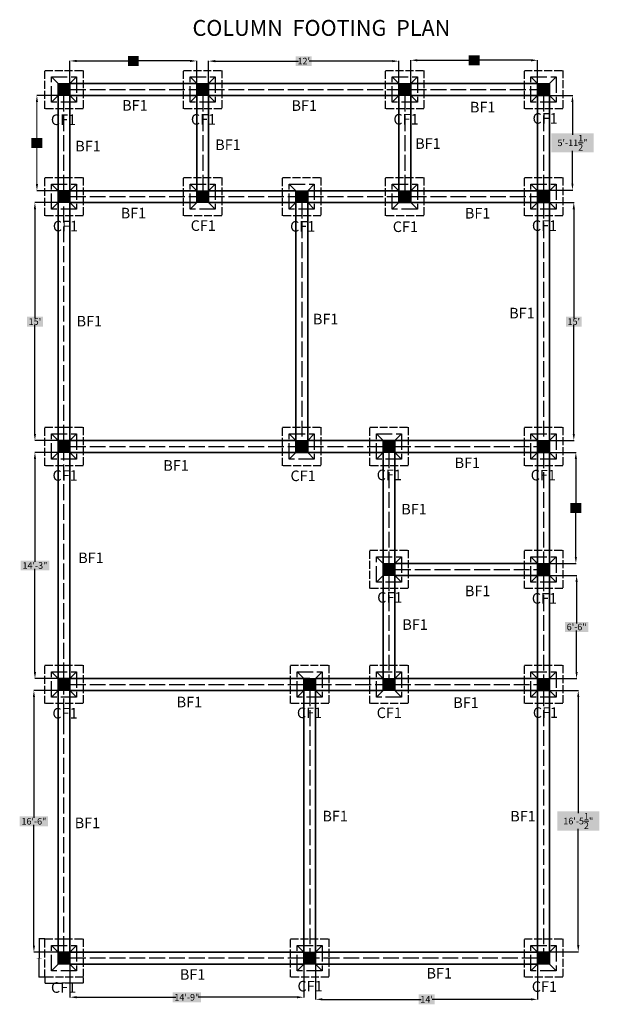
# Model space of a CAD drawing. Units: inches. Extents: x -8 to 1354, y -679 to 94.
# Tile 4 of 6: x 471 to 910, y -666 to 79. Entities that reach past the tile are written whole.
import ezdxf

# ---------------------------------------------------------------- set-up
doc = ezdxf.new("R2010")
doc.units = ezdxf.units.IN
doc.header["$MEASUREMENT"] = 0
doc.linetypes.add('ACAD_ISO02W100', pattern=[15, 12, -3])
for name, color, linetype, lineweight in [('A-ANNO-DIMS', 2, 'Continuous', 18), ('S-ANNO-TEXT', 7, 'Continuous', 25), ('S-BEAM', 152, 'Continuous', 35), ('S-FNDN', 3, 'ACAD_ISO02W100', 25), ('S-FNDN-PATT', 252, 'Continuous', 13)]:
    doc.layers.add(name, color=color, linetype=linetype, lineweight=lineweight)
doc.styles.get("Standard").update_dxf_attribs({"font": 'arial.ttf'})
doc.dimstyles.get("Standard").update_dxf_attribs({"dimtxt": 0.18, "dimasz": 0.18, "dimexe": 0.18, "dimexo": 0.0625, "dimgap": 0.09, "dimtad": 0, "dimtih": 1, "dimtoh": 1, "dimdec": 1, "dimzin": 0, "dimdsep": 46, "dimlunit": 4, "dimtxsty": 'Standard', "dimcen": 0.09, "dimclrd": 2, "dimclre": 3, "dimclrt": 6, "dimadec": 0, "dimazin": 0, "dimtfac": 1, "dimtdec": 1, "dimtofl": 0, "dimtmove": 0, "dimatfit": 3, "dimfxl": 1, "dimtfill": 2, "dimtfillclr": 4, "dimtolj": 1, "dimtzin": 0, "dimarcsym": 0})

# ---------------------------------------------------------------- blocks, each defined once
blk = doc.blocks.new('*D38')
at = {"layer": 'A-ANNO-DIMS', "color": 0, "lineweight": -2, "transparency": 16777216}
for p, q in [((509.02, 21.24), (509.02, 47.49)), ((514.02, 47.31), (554.62, 47.31)), ((600.02, 47.31), (559.41, 47.31)), ((605.02, 21.24), (605.02, 47.49))]:
    blk.add_line(p, q, dxfattribs=at)
at = {"layer": 'A-ANNO-DIMS', "color": 0, "transparency": 16777216}
for points in [[(514.02, 48.15), (514.02, 46.48), (509.02, 47.31)], [(600.02, 48.15), (600.02, 46.48), (605.02, 47.31)]]:
    blk.add_solid(points, dxfattribs=at)
at = {"layer": 'Defpoints', "color": 0, "transparency": 16777216}
for p in [(605.02, 47.31), (509.02, 21.17), (605.02, 21.17)]:
    blk.add_point(p, dxfattribs=at)
at = {"layer": 'A-ANNO-DIMS', "color": 0, "transparency": 16777216, "insert": (557.02, 47.31), "char_height": 5, "attachment_point": 5, "bg_fill": 1, "box_fill_scale": 1.25, "bg_fill_color": 4, "bg_fill_transparency": 0}
blk.add_mtext("\\A1;8'", dxfattribs=at)
blk = doc.blocks.new('*D39')
at = {"layer": 'A-ANNO-DIMS', "color": 0, "lineweight": -2, "transparency": 16777216}
for p, q in [((614.02, 21.24), (614.02, 47.35)), ((619.02, 47.17), (681.92, 47.17)), ((753.02, 47.17), (690.11, 47.17)), ((758.02, 21.24), (758.02, 47.35))]:
    blk.add_line(p, q, dxfattribs=at)
at = {"layer": 'A-ANNO-DIMS', "color": 0, "transparency": 16777216}
for points in [[(619.02, 48), (619.02, 46.33), (614.02, 47.17)], [(753.02, 48), (753.02, 46.33), (758.02, 47.17)]]:
    blk.add_solid(points, dxfattribs=at)
at = {"layer": 'Defpoints', "color": 0, "transparency": 16777216}
for p in [(758.02, 47.17), (614.02, 21.17), (758.02, 21.17)]:
    blk.add_point(p, dxfattribs=at)
at = {"layer": 'A-ANNO-DIMS', "color": 0, "transparency": 16777216, "insert": (686.02, 47.17), "char_height": 5, "attachment_point": 5, "bg_fill": 1, "box_fill_scale": 1.25, "bg_fill_color": 4, "bg_fill_transparency": 0}
blk.add_mtext("\\A1;12'", dxfattribs=at)
blk = doc.blocks.new('*D40')
at = {"layer": 'A-ANNO-DIMS', "color": 0, "lineweight": -2, "transparency": 16777216}
for p, q in [((767.02, 21.24), (767.02, 48.01)), ((772.02, 47.83), (812.62, 47.83)), ((858.02, 47.83), (817.41, 47.83)), ((863.02, 21.24), (863.02, 48.01))]:
    blk.add_line(p, q, dxfattribs=at)
at = {"layer": 'A-ANNO-DIMS', "color": 0, "transparency": 16777216}
for points in [[(772.02, 48.66), (772.02, 46.99), (767.02, 47.83)], [(858.02, 48.66), (858.02, 46.99), (863.02, 47.83)]]:
    blk.add_solid(points, dxfattribs=at)
at = {"layer": 'Defpoints', "color": 0, "transparency": 16777216}
for p in [(863.02, 47.83), (767.02, 21.17), (863.02, 21.17)]:
    blk.add_point(p, dxfattribs=at)
at = {"layer": 'A-ANNO-DIMS', "color": 0, "transparency": 16777216, "insert": (815.02, 47.83), "char_height": 5, "attachment_point": 5, "bg_fill": 1, "box_fill_scale": 1.25, "bg_fill_color": 4, "bg_fill_transparency": 0}
blk.add_mtext("\\A1;8'", dxfattribs=at)
blk = doc.blocks.new('*D41')
at = {"layer": 'A-ANNO-DIMS', "color": 0, "lineweight": -2, "transparency": 16777216}
for p, q in [((508.95, 21.17), (483.84, 21.17)), ((508.95, -50.83), (483.84, -50.83))]:
    blk.add_line(p, q, dxfattribs=at)
at = {"layer": 'A-ANNO-DIMS', "color": 0, "lineweight": 5, "transparency": 16777216}
for p, q in [((484.02, 16.17), (484.02, -12.18)), ((484.02, -45.83), (484.02, -17.47))]:
    blk.add_line(p, q, dxfattribs=at)
at = {"layer": 'A-ANNO-DIMS', "color": 0, "transparency": 16777216}
for points in [[(483.19, 16.17), (484.85, 16.17), (484.02, 21.17)], [(483.19, -45.83), (484.85, -45.83), (484.02, -50.83)]]:
    blk.add_solid(points, dxfattribs=at)
at = {"layer": 'Defpoints', "color": 0, "transparency": 16777216}
for p in [(484.02, 21.17), (509.02, 21.17), (509.02, -50.83)]:
    blk.add_point(p, dxfattribs=at)
at = {"layer": 'A-ANNO-DIMS', "color": 0, "transparency": 16777216, "insert": (484.02, -14.83), "char_height": 5, "attachment_point": 5, "bg_fill": 1, "box_fill_scale": 1.25, "bg_fill_color": 4, "bg_fill_transparency": 0}
blk.add_mtext("\\A1;6'", dxfattribs=at)
blk = doc.blocks.new('*D42')
at = {"layer": 'A-ANNO-DIMS', "color": 0, "lineweight": -2, "transparency": 16777216}
for p, q in [((863.08, 21.17), (889.6, 21.17)), ((889.42, 16.17), (889.42, -8.63)), ((889.42, -45.4), (889.42, -20.6)), ((863.08, -50.4), (889.6, -50.4))]:
    blk.add_line(p, q, dxfattribs=at)
at = {"layer": 'A-ANNO-DIMS', "color": 0, "transparency": 16777216}
for points in [[(888.58, 16.17), (890.25, 16.17), (889.42, 21.17)], [(888.58, -45.4), (890.25, -45.4), (889.42, -50.4)]]:
    blk.add_solid(points, dxfattribs=at)
at = {"layer": 'Defpoints', "color": 0, "transparency": 16777216}
for p in [(863.02, 21.17), (863.02, -50.4), (889.42, -50.4)]:
    blk.add_point(p, dxfattribs=at)
at = {"layer": 'A-ANNO-DIMS', "color": 0, "transparency": 16777216, "insert": (889.42, -14.61), "char_height": 5, "attachment_point": 5, "bg_fill": 1, "box_fill_scale": 1.25, "bg_fill_color": 4, "bg_fill_transparency": 0}
blk.add_mtext('\\A1;5\'-11{\\H1x;\\S1/2;}"', dxfattribs=at)
blk = doc.blocks.new('*D43')
at = {"layer": 'A-ANNO-DIMS', "color": 0, "lineweight": -2, "transparency": 16777216}
for p, q in [((508.95, -59.83), (482.33, -59.83)), ((482.51, -64.83), (482.51, -147.18)), ((482.51, -234.83), (482.51, -152.47)), ((508.95, -239.83), (482.33, -239.83))]:
    blk.add_line(p, q, dxfattribs=at)
at = {"layer": 'A-ANNO-DIMS', "color": 0, "transparency": 16777216}
for points in [[(481.68, -64.83), (483.34, -64.83), (482.51, -59.83)], [(481.68, -234.83), (483.34, -234.83), (482.51, -239.83)]]:
    blk.add_solid(points, dxfattribs=at)
at = {"layer": 'Defpoints', "color": 0, "transparency": 16777216}
for p in [(509.02, -59.83), (482.51, -239.83), (509.02, -239.83)]:
    blk.add_point(p, dxfattribs=at)
at = {"layer": 'A-ANNO-DIMS', "color": 0, "transparency": 16777216, "insert": (482.51, -149.83), "char_height": 5, "attachment_point": 5, "bg_fill": 1, "box_fill_scale": 1.25, "bg_fill_color": 4, "bg_fill_transparency": 0}
blk.add_mtext("\\A1;15'", dxfattribs=at)
blk = doc.blocks.new('*D44')
at = {"layer": 'A-ANNO-DIMS', "color": 0, "lineweight": -2, "transparency": 16777216}
for p, q in [((863.08, -59.83), (890.63, -59.83)), ((890.45, -64.83), (890.45, -147.18)), ((890.45, -234.83), (890.45, -152.47)), ((863.08, -239.83), (890.63, -239.83))]:
    blk.add_line(p, q, dxfattribs=at)
at = {"layer": 'A-ANNO-DIMS', "color": 0, "transparency": 16777216}
for points in [[(889.61, -64.83), (891.28, -64.83), (890.45, -59.83)], [(889.61, -234.83), (891.28, -234.83), (890.45, -239.83)]]:
    blk.add_solid(points, dxfattribs=at)
at = {"layer": 'Defpoints', "color": 0, "transparency": 16777216}
for p in [(863.02, -59.83), (863.02, -239.83), (890.45, -239.83)]:
    blk.add_point(p, dxfattribs=at)
at = {"layer": 'A-ANNO-DIMS', "color": 0, "transparency": 16777216, "insert": (890.45, -149.83), "char_height": 5, "attachment_point": 5, "bg_fill": 1, "box_fill_scale": 1.25, "bg_fill_color": 4, "bg_fill_transparency": 0}
blk.add_mtext("\\A1;15'", dxfattribs=at)
blk = doc.blocks.new('*D45')
at = {"layer": 'A-ANNO-DIMS', "color": 0, "lineweight": -2, "transparency": 16777216}
for p, q in [((863.08, -248.83), (892.19, -248.83)), ((892.01, -253.83), (892.01, -288.24)), ((892.01, -327.83), (892.01, -293.42)), ((863.08, -332.83), (892.19, -332.83))]:
    blk.add_line(p, q, dxfattribs=at)
at = {"layer": 'A-ANNO-DIMS', "color": 0, "transparency": 16777216}
for points in [[(891.18, -253.83), (892.85, -253.83), (892.01, -248.83)], [(891.18, -327.83), (892.85, -327.83), (892.01, -332.83)]]:
    blk.add_solid(points, dxfattribs=at)
at = {"layer": 'Defpoints', "color": 0, "transparency": 16777216}
for p in [(863.02, -248.83), (863.02, -332.83), (892.01, -332.83)]:
    blk.add_point(p, dxfattribs=at)
at = {"layer": 'A-ANNO-DIMS', "color": 0, "transparency": 16777216, "insert": (892.01, -290.83), "char_height": 5, "attachment_point": 5, "bg_fill": 1, "box_fill_scale": 1.25, "bg_fill_color": 4, "bg_fill_transparency": 0}
blk.add_mtext("\\A1;7'", dxfattribs=at)
blk = doc.blocks.new('*D46')
at = {"layer": 'A-ANNO-DIMS', "color": 0, "lineweight": -2, "transparency": 16777216}
for p, q in [((863.08, -341.83), (892.75, -341.83)), ((892.57, -346.83), (892.57, -378.18)), ((892.57, -414.83), (892.57, -383.47)), ((863.08, -419.83), (892.75, -419.83))]:
    blk.add_line(p, q, dxfattribs=at)
at = {"layer": 'A-ANNO-DIMS', "color": 0, "transparency": 16777216}
for points in [[(891.73, -346.83), (893.4, -346.83), (892.57, -341.83)], [(891.73, -414.83), (893.4, -414.83), (892.57, -419.83)]]:
    blk.add_solid(points, dxfattribs=at)
at = {"layer": 'Defpoints', "color": 0, "transparency": 16777216}
for p in [(863.02, -341.83), (892.57, -341.83), (863.02, -419.83)]:
    blk.add_point(p, dxfattribs=at)
at = {"layer": 'A-ANNO-DIMS', "color": 0, "transparency": 16777216, "insert": (892.57, -380.83), "char_height": 5, "attachment_point": 5, "bg_fill": 1, "box_fill_scale": 1.25, "bg_fill_color": 4, "bg_fill_transparency": 0}
blk.add_mtext('\\A1;6\'-6"', dxfattribs=at)
blk = doc.blocks.new('*D47')
at = {"layer": 'A-ANNO-DIMS', "color": 0, "lineweight": -2, "transparency": 16777216}
for p, q in [((863.08, -428.83), (894, -428.83)), ((893.82, -433.83), (893.82, -521.69)), ((893.82, -621.52), (893.82, -533.66)), ((863.08, -626.52), (894, -626.52))]:
    blk.add_line(p, q, dxfattribs=at)
at = {"layer": 'A-ANNO-DIMS', "color": 0, "transparency": 16777216}
for points in [[(892.98, -433.83), (894.65, -433.83), (893.82, -428.83)], [(892.98, -621.52), (894.65, -621.52), (893.82, -626.52)]]:
    blk.add_solid(points, dxfattribs=at)
at = {"layer": 'Defpoints', "color": 0, "transparency": 16777216}
for p in [(863.02, -428.83), (863.02, -626.52), (893.82, -626.52)]:
    blk.add_point(p, dxfattribs=at)
at = {"layer": 'A-ANNO-DIMS', "color": 0, "transparency": 16777216, "insert": (893.82, -527.67), "char_height": 5, "attachment_point": 5, "bg_fill": 1, "box_fill_scale": 1.25, "bg_fill_color": 4, "bg_fill_transparency": 0}
blk.add_mtext('\\A1;16\'-5{\\H1x;\\S1/2;}"', dxfattribs=at)
blk = doc.blocks.new('*D48')
at = {"layer": 'A-ANNO-DIMS', "color": 0, "lineweight": -2, "transparency": 16777216}
for p, q in [((508.95, -248.83), (482.35, -248.83)), ((482.53, -253.83), (482.53, -331.68)), ((482.53, -414.83), (482.53, -336.97)), ((508.95, -419.83), (482.35, -419.83))]:
    blk.add_line(p, q, dxfattribs=at)
at = {"layer": 'A-ANNO-DIMS', "color": 0, "transparency": 16777216}
for points in [[(481.69, -253.83), (483.36, -253.83), (482.53, -248.83)], [(481.69, -414.83), (483.36, -414.83), (482.53, -419.83)]]:
    blk.add_solid(points, dxfattribs=at)
at = {"layer": 'Defpoints', "color": 0, "transparency": 16777216}
for p in [(509.02, -248.83), (482.53, -419.83), (509.02, -419.83)]:
    blk.add_point(p, dxfattribs=at)
at = {"layer": 'A-ANNO-DIMS', "color": 0, "transparency": 16777216, "insert": (482.53, -334.33), "char_height": 5, "attachment_point": 5, "bg_fill": 1, "box_fill_scale": 1.25, "bg_fill_color": 4, "bg_fill_transparency": 0}
blk.add_mtext('\\A1;14\'-3"', dxfattribs=at)
blk = doc.blocks.new('*D49')
at = {"layer": 'A-ANNO-DIMS', "color": 0, "lineweight": -2, "transparency": 16777216}
for p, q in [((508.95, -428.83), (481.56, -428.83)), ((481.74, -433.83), (481.74, -525.18)), ((481.74, -621.83), (481.74, -530.47)), ((508.95, -626.83), (481.56, -626.83))]:
    blk.add_line(p, q, dxfattribs=at)
at = {"layer": 'A-ANNO-DIMS', "color": 0, "transparency": 16777216}
for points in [[(480.91, -433.83), (482.57, -433.83), (481.74, -428.83)], [(480.91, -621.83), (482.57, -621.83), (481.74, -626.83)]]:
    blk.add_solid(points, dxfattribs=at)
at = {"layer": 'Defpoints', "color": 0, "transparency": 16777216}
for p in [(509.02, -428.83), (481.74, -626.83), (509.02, -626.83)]:
    blk.add_point(p, dxfattribs=at)
at = {"layer": 'A-ANNO-DIMS', "color": 0, "transparency": 16777216, "insert": (481.74, -527.83), "char_height": 5, "attachment_point": 5, "bg_fill": 1, "box_fill_scale": 1.25, "bg_fill_color": 4, "bg_fill_transparency": 0}
blk.add_mtext('\\A1;16\'-6"', dxfattribs=at)
blk = doc.blocks.new('*D50')
at = {"layer": 'A-ANNO-DIMS', "color": 0, "lineweight": -2, "transparency": 16777216}
for p, q in [((509.02, -626.89), (509.02, -661.09)), ((686.02, -626.89), (686.02, -661.09)), ((514.02, -660.91), (589.07, -660.91)), ((681.02, -660.91), (605.96, -660.91))]:
    blk.add_line(p, q, dxfattribs=at)
at = {"layer": 'A-ANNO-DIMS', "color": 0, "transparency": 16777216}
for points in [[(514.02, -660.07), (514.02, -661.74), (509.02, -660.91)], [(681.02, -660.07), (681.02, -661.74), (686.02, -660.91)]]:
    blk.add_solid(points, dxfattribs=at)
at = {"layer": 'Defpoints', "color": 0, "transparency": 16777216}
for p in [(509.02, -626.83), (686.02, -626.83), (686.02, -660.91)]:
    blk.add_point(p, dxfattribs=at)
at = {"layer": 'A-ANNO-DIMS', "color": 0, "transparency": 16777216, "insert": (597.52, -660.91), "char_height": 5, "attachment_point": 5, "bg_fill": 1, "box_fill_scale": 1.25, "bg_fill_color": 4, "bg_fill_transparency": 0}
blk.add_mtext('\\A1;14\'-9"', dxfattribs=at)
blk = doc.blocks.new('*D51')
at = {"layer": 'A-ANNO-DIMS', "color": 0, "lineweight": -2, "transparency": 16777216}
for p, q in [((695.02, -626.89), (695.02, -662.7)), ((863.02, -626.89), (863.02, -662.7))]:
    blk.add_line(p, q, dxfattribs=at)
at = {"layer": 'A-ANNO-DIMS', "color": 0, "lineweight": 25, "transparency": 16777216}
for p, q in [((700.02, -662.52), (774.92, -662.52)), ((858.02, -662.52), (783.11, -662.52))]:
    blk.add_line(p, q, dxfattribs=at)
at = {"layer": 'A-ANNO-DIMS', "color": 0, "transparency": 16777216}
for points in [[(700.02, -661.68), (700.02, -663.35), (695.02, -662.52)], [(858.02, -661.68), (858.02, -663.35), (863.02, -662.52)]]:
    blk.add_solid(points, dxfattribs=at)
at = {"layer": 'Defpoints', "color": 0, "transparency": 16777216}
for p in [(695.02, -626.83), (863.02, -626.83), (863.02, -662.52)]:
    blk.add_point(p, dxfattribs=at)
at = {"layer": 'A-ANNO-DIMS', "color": 0, "transparency": 16777216, "insert": (779.02, -662.52), "char_height": 5, "attachment_point": 5, "bg_fill": 1, "box_fill_scale": 1.25, "bg_fill_color": 4, "bg_fill_transparency": 0}
blk.add_mtext("\\A1;14'", dxfattribs=at)
blk = doc.blocks.new('COLUMN-FOOTING-CF1')
at = {"ltscale": 0.5}
for p, q in [((0, 0), (0, 29)), ((0, 29), (29, 29)), ((29, 29), (29, 0)), ((29, 0), (0, 0))]:
    blk.add_line(p, q, dxfattribs=at)
for p, q in [((5, 5), (5, 24)), ((5, 24), (24, 24)), ((10, 19), (5, 24)), ((19, 19), (24, 24)), ((24, 24), (24, 5)), ((10, 10), (10, 19)), ((10, 19), (19, 19)), ((19, 19), (19, 10)), ((5, 5), (10, 10)), ((19, 10), (10, 10)), ((24, 5), (19, 10)), ((24, 5), (5, 5))]:
    blk.add_line(p, q)
blk = doc.blocks.new('*D77')
at = {"layer": 'A-ANNO-DIMS', "color": 3, "lineweight": -2, "transparency": 16777216}
for p, q in [((489.95, -616.83), (485.49, -616.83)), ((489.95, -645.83), (485.49, -645.83))]:
    blk.add_line(p, q, dxfattribs=at)
at = {"layer": 'A-ANNO-DIMS', "color": 2, "lineweight": -2, "transparency": 16777216}
for p, q in [((485.67, -617.01), (485.67, -631.14)), ((485.67, -645.65), (485.67, -631.51))]:
    blk.add_line(p, q, dxfattribs=at)
at = {"layer": 'A-ANNO-DIMS', "color": 2, "transparency": 16777216}
for points in [[(485.64, -617.01), (485.7, -617.01), (485.67, -616.83)], [(485.64, -645.65), (485.7, -645.65), (485.67, -645.83)]]:
    blk.add_solid(points, dxfattribs=at)
at = {"layer": 'Defpoints', "color": 0, "transparency": 16777216}
for p in [(490.02, -616.83), (485.67, -645.83), (490.02, -645.83)]:
    blk.add_point(p, dxfattribs=at)
at = {"layer": 'A-ANNO-DIMS', "color": 6, "transparency": 16777216, "insert": (485.67, -631.33), "char_height": 0.18, "attachment_point": 5, "bg_fill": 1, "box_fill_scale": 1.25, "bg_fill_color": 4, "bg_fill_transparency": 0}
blk.add_mtext('\\A1;COLUMN FOOTING CF1 2\'-5" TYP.', dxfattribs=at)
blk = doc.blocks.new('*D78')
at = {"layer": 'A-ANNO-DIMS', "color": 3, "lineweight": -2, "transparency": 16777216}
for p, q in [((490.02, -645.89), (490.02, -650.36)), ((519.02, -645.89), (519.02, -650.36))]:
    blk.add_line(p, q, dxfattribs=at)
at = {"layer": 'A-ANNO-DIMS', "color": 2, "lineweight": -2, "transparency": 16777216}
for p, q in [((490.2, -650.18), (503.88, -650.18)), ((518.84, -650.18), (505.16, -650.18))]:
    blk.add_line(p, q, dxfattribs=at)
at = {"layer": 'A-ANNO-DIMS', "color": 2, "transparency": 16777216}
for points in [[(490.2, -650.15), (490.2, -650.21), (490.02, -650.18)], [(518.84, -650.15), (518.84, -650.21), (519.02, -650.18)]]:
    blk.add_solid(points, dxfattribs=at)
at = {"layer": 'Defpoints', "color": 0, "transparency": 16777216}
for p in [(490.02, -645.83), (519.02, -645.83), (519.02, -650.18)]:
    blk.add_point(p, dxfattribs=at)
at = {"layer": 'A-ANNO-DIMS', "color": 6, "transparency": 16777216, "insert": (504.52, -650.18), "char_height": 0.18, "attachment_point": 5, "bg_fill": 1, "box_fill_scale": 1.25, "bg_fill_color": 4, "bg_fill_transparency": 0}
blk.add_mtext('\\A1;2\'-5" TYP.', dxfattribs=at)

msp = doc.modelspace()

# ---------------------------------------------------------------- hatches: boundary and pattern name
at = {"layer": 'S-FNDN-PATT'}
h = msp.add_hatch(dxfattribs=at)
h.set_pattern_fill('ANSI31', color=256)
h.set_pattern_definition([(45, (-15.72023, 0), (-0.088388348, 0.088388348), [])])
h.paths.add_polyline_path([(509.02, 30.17), (500.02, 30.17), (500.02, 21.17), (509.02, 21.17)])
h.paths.add_polyline_path([(614.02, 30.17), (605.02, 30.17), (605.02, 21.17), (614.02, 21.17)])
h.paths.add_polyline_path([(767.02, 30.17), (758.02, 30.17), (758.02, 21.17), (767.02, 21.17)])
h.paths.add_polyline_path([(863.02, 30.17), (863.02, 21.17), (872.02, 21.17), (872.02, 30.17)])
h.paths.add_polyline_path([(509.02, -59.83), (509.02, -50.83), (500.02, -50.83), (500.02, -59.83)])
h.paths.add_polyline_path([(605.02, -59.83), (614.02, -59.83), (614.02, -50.83), (605.02, -50.83)])
h.paths.add_polyline_path([(689.02, -50.83), (680.02, -50.83), (680.02, -59.83), (689.02, -59.83)])
h.paths.add_polyline_path([(767.02, -50.83), (758.02, -50.83), (758.02, -59.83), (767.02, -59.83)])
h.paths.add_polyline_path([(863.02, -59.83), (872.02, -59.83), (872.02, -50.83), (863.02, -50.83)])
h.paths.add_polyline_path([(500.02, -248.83), (509.02, -248.83), (509.02, -239.83), (500.02, -239.83)])
h.paths.add_polyline_path([(680.02, -239.83), (680.02, -248.83), (689.02, -248.83), (689.02, -239.83)])
h.paths.add_polyline_path([(746.02, -239.83), (746.02, -248.83), (755.02, -248.83), (755.02, -239.83)])
h.paths.add_polyline_path([(872.02, -248.83), (872.02, -239.83), (863.02, -239.83), (863.02, -248.83)])
h.paths.add_polyline_path([(746.02, -332.83), (746.02, -341.83), (755.02, -341.83), (755.02, -332.83)])
h.paths.add_polyline_path([(863.02, -332.83), (863.02, -341.83), (872.02, -341.83), (872.02, -332.83)])
h.paths.add_polyline_path([(863.02, -428.83), (872.02, -428.83), (872.02, -419.83), (863.02, -419.83)])
h.paths.add_polyline_path([(755.02, -419.83), (746.02, -419.83), (746.02, -428.83), (755.02, -428.83)])
h.paths.add_polyline_path([(695.02, -419.83), (686.02, -419.83), (686.02, -428.83), (695.02, -428.83)])
h.paths.add_polyline_path([(509.02, -419.83), (500.02, -419.83), (500.02, -428.83), (509.02, -428.83)])
h.paths.add_polyline_path([(500.02, -626.83), (500.02, -635.83), (509.02, -635.83), (509.02, -626.83)])
h.paths.add_polyline_path([(695.02, -626.83), (686.02, -626.83), (686.02, -635.83), (695.02, -635.83)])
h.paths.add_polyline_path([(863.02, -626.83), (863.02, -635.83), (872.02, -635.83), (872.02, -626.83)])

# ---------------------------------------------------------------- linework, layer by layer
at = {"layer": 'S-BEAM'}
for p, q in [((509.02, 30.17), (605.02, 30.17)), ((614.02, 30.17), (758.02, 30.17)), ((767.02, 30.17), (863.02, 30.17)), ((500.02, -50.83), (500.02, 21.17)), ((509.02, 21.17), (605.02, 21.17)), ((509.02, -50.83), (509.02, 21.17)), ((605.02, 21.17), (605.02, -50.83)), ((614.02, 21.17), (614.02, -50.83)), ((614.02, 21.17), (758.02, 21.17)), ((758.02, 21.17), (758.02, -50.83)), ((767.02, 21.17), (767.02, -50.83)), ((767.02, 21.17), (863.02, 21.17)), ((863.02, 21.17), (863.02, -50.83)), ((872.02, 21.17), (872.02, -239.83)), ((872.02, 21.17), (872.02, -50.83)), ((605.02, -50.83), (509.02, -50.83)), ((680.02, -50.83), (614.02, -50.83)), ((758.02, -50.83), (689.02, -50.83)), ((863.02, -50.83), (767.02, -50.83)), ((500.02, -59.83), (500.02, -635.83)), ((605.02, -59.83), (509.02, -59.83)), ((509.02, -59.83), (509.02, -239.83)), ((680.02, -59.83), (614.02, -59.83)), ((680.02, -239.83), (680.02, -59.83)), ((767.02, -59.83), (689.02, -59.83)), ((689.02, -239.83), (689.02, -59.83)), ((863.02, -59.83), (767.02, -59.83)), ((863.02, -59.83), (863.02, -239.83)), ((509.02, -239.83), (680.02, -239.83)), ((689.02, -239.83), (863.02, -239.83)), ((509.02, -248.83), (509.02, -419.83)), ((509.02, -248.83), (554.02, -248.83)), ((684.52, -248.83), (509.02, -248.83)), ((554.02, -248.83), (640.47, -248.83)), ((746.02, -248.83), (684.52, -248.83)), ((729.02, -248.83), (746.02, -248.83)), ((746.02, -419.83), (746.02, -248.83)), ((755.02, -248.83), (863.02, -248.83)), ((755.02, -332.83), (755.02, -248.83)), ((863.02, -248.83), (863.02, -332.83)), ((872.02, -248.83), (872.02, -341.83)), ((863.02, -332.83), (755.02, -332.83)), ((755.02, -419.83), (755.02, -341.83)), ((863.02, -341.83), (755.11, -341.83)), ((863.02, -341.83), (863.02, -419.83)), ((872.02, -341.83), (872.02, -428.83)), ((690.52, -419.83), (509.02, -419.83)), ((746.02, -419.83), (695.02, -419.83)), ((863.02, -419.83), (755.11, -419.83)), ((509.02, -428.83), (509.02, -626.83)), ((686.02, -428.83), (509.02, -428.83)), ((686.02, -626.83), (686.02, -428.83)), ((746.02, -428.83), (695.02, -428.83)), ((695.02, -626.83), (695.02, -428.83)), ((863.02, -428.83), (755.02, -428.83)), ((863.02, -428.83), (826.28, -428.83)), ((863.02, -428.83), (863.02, -626.83)), ((872.02, -428.83), (872.02, -626.83)), ((686.02, -626.83), (509.02, -626.83)), ((863.02, -626.83), (695.02, -626.83)), ((686.02, -635.83), (509.02, -635.83)), ((863.02, -635.83), (695.02, -635.83))]:
    msp.add_line(p, q, dxfattribs=at)
at = {"layer": 'S-FNDN'}
for p, q in [((509.02, 25.67), (605.02, 25.67)), ((614.02, 25.67), (758.02, 25.67)), ((767.02, 25.67), (863.02, 25.67)), ((504.52, -50.83), (504.52, 21.17)), ((609.52, 21.17), (609.52, -50.83)), ((762.52, 21.17), (762.52, -50.83)), ((867.52, 21.17), (867.52, -50.83)), ((509.02, -55.33), (605.02, -55.33)), ((614.02, -55.33), (680.02, -55.33)), ((689.02, -55.33), (758.02, -55.33)), ((767.02, -55.33), (863.02, -55.33)), ((504.52, -239.83), (504.52, -59.83)), ((684.52, -59.83), (684.52, -239.83)), ((867.52, -59.83), (867.52, -239.83)), ((509.02, -244.33), (680.02, -244.33)), ((689.02, -244.33), (746.02, -244.33)), ((755.02, -244.33), (863.02, -244.33)), ((504.52, -419.83), (504.52, -248.83)), ((750.52, -248.83), (750.52, -332.83)), ((867.52, -248.83), (867.52, -332.83)), ((750.52, -341.83), (750.52, -419.83)), ((755.02, -337.33), (863.02, -337.33)), ((867.52, -341.83), (867.52, -419.83)), ((509.02, -424.33), (686.02, -424.33)), ((695.02, -424.33), (746.02, -424.33)), ((755.02, -424.33), (863.02, -424.33)), ((504.52, -626.83), (504.52, -428.83)), ((690.52, -428.83), (690.52, -626.83)), ((867.52, -428.83), (867.52, -626.83)), ((686.02, -631.33), (509.02, -631.33)), ((863.02, -631.33), (695.02, -631.33))]:
    msp.add_line(p, q, dxfattribs=at)

# ---------------------------------------------------------------- block references
for p, rotation in [((519.02, 11.17), 89.99999999999935), ((624.02, 11.17), 90), ((777.02, 11.17), 90.00000000000045), ((882.02, 11.17), 90.00000000000067), ((519.02, -40.83), 180), ((595.02, -40.83), 269.9999999999999), ((699.02, -69.83), 90.0000000000003), ((748.02, -40.83), 269.9999999999995), ((519.02, -229.83), 180), ((670.02, -229.83), 269.9999999999996), ((765.02, -258.83), 90.00000000000033), ((882.02, -229.83), 180), ((765.02, -322.83), 179.9941756767035), ((490.02, -409.83), 270.0000000000007), ((705.02, -438.83), 90.00000000000021), ((736.02, -409.82), 269.9941744923129), ((882.02, -409.83), 180), ((490.02, -616.83), 270.0000000000009), ((676.02, -616.83), 269.9999999999993), ((853.02, -616.83), 270)]:
    msp.add_blockref('COLUMN-FOOTING-CF1', p, dxfattribs=dict(at, rotation=rotation))
for p in [(853.02, -69.83), (853.02, -351.83)]:
    msp.add_blockref('COLUMN-FOOTING-CF1', p, dxfattribs=at)

# ---------------------------------------------------------------- texts
at = {"layer": 'S-ANNO-TEXT', "attachment_point": 1}
for s, width, heights, insert, char_height in [('COLUMN  FOOTING  PLAN', 250.6777, [12.42], (601.8, 78.3), 12), ('BF1', 71.0443, [0], (548.56, 17.7), 8), ('BF1', 71.0443, [0], (676.75, 17.55), 8), ('BF1', 71.0443, [0], (811.86, 16.39), 8), ('CF1', 71.0443, [0], (859.22, 7.84), 8), ('CF1', 71.0443, [0], (494.6, 6.85), 8), ('CF1', 71.0443, [0], (600.59, 7.11), 8), ('CF1', 71.0443, [0], (753.9, 7.21), 8), ('BF1', 71.0443, [0], (513.1, -13.09), 8), ('BF1', 71.0443, [0], (619.01, -12.09), 8), ('BF1', 71.0443, [0], (770.4, -11.18), 8), ('BF1', 71.0443, [0], (547.47, -63.77), 8), ('BF1', 71.0443, [0], (808.01, -63.88), 8), ('CF1', 71.0443, [0], (496.08, -73.62), 8), ('CF1', 71.0443, [0], (600.42, -73.25), 8), ('CF1', 71.0443, [0], (675.68, -73.81), 8), ('CF1', 71.0443, [0], (753.42, -74.09), 8), ('CF1', 71.0443, [0], (858.75, -73.27), 8), ('BF1', 71.0443, [0], (841.51, -139.42), 8), ('BF1', 71.0443, [0], (514.06, -145.5), 8), ('BF1', 71.0443, [0], (692.99, -143.92), 8), ('BF1', 71.0443, [0], (800.24, -252.67), 8), ('BF1', 71.0443, [0], (579.73, -254.66), 8), ('CF1', 71.0443, [0], (495.83, -262.26), 8), ('CF1', 71.0443, [0], (675.97, -262.5), 8), ('CF1', 71.0443, [0], (741.25, -261.83), 8), ('CF1', 71.0443, [0], (857.83, -261.99), 8), ('BF1', 71.0443, [0], (759.87, -287.71), 8), ('BF1', 71.0443, [0], (515.26, -324.55), 8), ('BF1', 71.0443, [0], (808.03, -349.58), 8), ('CF1', 71.0443, [0], (741.63, -354.5), 8), ('CF1', 71.0443, [0], (858.66, -355.21), 8), ('BF1', 71.0443, [0], (760.67, -375.02), 8), ('BF1', 71.0443, [0], (589.83, -433.61), 8), ('BF1', 71.0443, [0], (799.23, -434.09), 8), ('CF1', 71.0443, [0], (495.75, -442.1), 8), ('CF1', 71.0443, [0], (680.84, -441.79), 8), ('CF1', 71.0443, [0], (741.25, -441.77), 8), ('CF1', 71.0443, [0], (859.44, -441.63), 8), ('BF1', 71.0443, [0], (700.16, -519.88), 8), ('BF1', 71.0443, [0], (842.38, -519.98), 8), ('BF1', 71.0443, [0], (512.63, -525.05), 8), ('BF1', 71.0443, [0], (592.25, -639.7), 8), ('BF1', 71.0443, [0], (778.94, -638.77), 8), ('CF1', 71.0443, [0], (494.67, -649.56), 8), ('CF1', 71.0443, [0], (681.27, -648.53), 8), ('CF1', 71.0443, [0], (858.65, -648.89), 8)]:
    msp.add_mtext_dynamic_manual_height_columns(s, width=width, gutter_width=1, heights=heights, dxfattribs=dict(at, insert=insert, char_height=char_height))

# ---------------------------------------------------------------- dimensions: what is measured, and where the dimension line sits
at = {"layer": 'A-ANNO-DIMS'}
for base, p1, p2, override, picture, middle in [((605.02, 47.31), (509.02, 21.17), (605.02, 21.17), {"dimtxt": 5, "dimasz": 5, "dimclrd": 0, "dimclre": 0, "dimclrt": 0}, '*D38', (557.02, 47.31)), ((758.02, 47.17), (614.02, 21.17), (758.02, 21.17), {"dimtxt": 5, "dimasz": 5, "dimclrd": 0, "dimclre": 0, "dimclrt": 0}, '*D39', (686.02, 47.17)), ((863.02, 47.83), (767.02, 21.17), (863.02, 21.17), {"dimtxt": 5, "dimasz": 5, "dimclrd": 0, "dimclre": 0, "dimclrt": 0}, '*D40', (815.02, 47.83)), ((686.02, -660.91), (509.02, -626.83), (686.02, -626.83), {"dimtxt": 5, "dimasz": 5, "dimclrd": 0, "dimclre": 0, "dimclrt": 0}, '*D50', (597.52, -660.91)), ((863.02, -662.52), (695.02, -626.83), (863.02, -626.83), {"dimtxt": 5, "dimasz": 5, "dimclrd": 0, "dimclre": 0, "dimclrt": 0, "dimlwd": 25}, '*D51', (779.02, -662.52))]:
    dim = msp.add_linear_dim(base=base, p1=p1, p2=p2, dimstyle='Standard', override=override, dxfattribs=at)
    dim.commit()
    dim.dimension.update_dxf_attribs({"geometry": picture, "text_midpoint": middle})
for base, p1, p2, override, picture, middle in [((484.02, 21.17), (509.02, -50.83), (509.02, 21.17), {"dimtxt": 5, "dimasz": 5, "dimclrd": 0, "dimclre": 0, "dimclrt": 0, "dimlwd": 5}, '*D41', (484.02, -14.83)), ((889.42, -50.4), (863.02, 21.17), (863.02, -50.4), {"dimtxt": 5, "dimasz": 5, "dimclrd": 0, "dimclre": 0, "dimclrt": 0}, '*D42', (889.42, -14.61)), ((482.51, -239.83), (509.02, -59.83), (509.02, -239.83), {"dimtxt": 5, "dimasz": 5, "dimclrd": 0, "dimclre": 0, "dimclrt": 0}, '*D43', (482.51, -149.83)), ((890.45, -239.83), (863.02, -59.83), (863.02, -239.83), {"dimtxt": 5, "dimasz": 5, "dimclrd": 0, "dimclre": 0, "dimclrt": 0}, '*D44', (890.45, -149.83)), ((482.53, -419.83), (509.02, -248.83), (509.02, -419.83), {"dimtxt": 5, "dimasz": 5, "dimclrd": 0, "dimclre": 0, "dimclrt": 0}, '*D48', (482.53, -334.33)), ((892.01, -332.83), (863.02, -248.83), (863.02, -332.83), {"dimtxt": 5, "dimasz": 5, "dimclrd": 0, "dimclre": 0, "dimclrt": 0}, '*D45', (892.01, -290.83)), ((892.57, -341.83), (863.02, -419.83), (863.02, -341.83), {"dimtxt": 5, "dimasz": 5, "dimclrd": 0, "dimclre": 0, "dimclrt": 0}, '*D46', (892.57, -380.83)), ((481.74, -626.83), (509.02, -428.83), (509.02, -626.83), {"dimtxt": 5, "dimasz": 5, "dimclrd": 0, "dimclre": 0, "dimclrt": 0}, '*D49', (481.74, -527.83)), ((893.82, -626.52), (863.02, -428.83), (863.02, -626.52), {"dimtxt": 5, "dimasz": 5, "dimclrd": 0, "dimclre": 0, "dimclrt": 0}, '*D47', (893.82, -527.67))]:
    dim = msp.add_linear_dim(base=base, p1=p1, p2=p2, angle=90, dimstyle='Standard', override=override, dxfattribs=at)
    dim.commit()
    dim.dimension.update_dxf_attribs({"geometry": picture, "text_midpoint": middle})
for base, p1, p2, angle, text, picture, middle in [((485.67, -645.83), (490.02, -616.83), (490.02, -645.83), 270, 'COLUMN FOOTING CF1 <> TYP.', '*D77', (485.67, -631.33)), ((519.02, -650.18), (490.02, -645.83), (519.02, -645.83), 0, '<> TYP.', '*D78', (504.52, -650.18))]:
    dim = msp.add_linear_dim(base=base, p1=p1, p2=p2, angle=angle, text=text, dimstyle='Standard', override={"dimdec": 1, "dimrnd": 0, "dimzin": 1, "dimlunit": 4, "dimfrac": 2}, dxfattribs=at)
    dim.commit()
    dim.dimension.update_dxf_attribs({"geometry": picture, "text_midpoint": middle})

doc.saveas('drawing.dxf')
